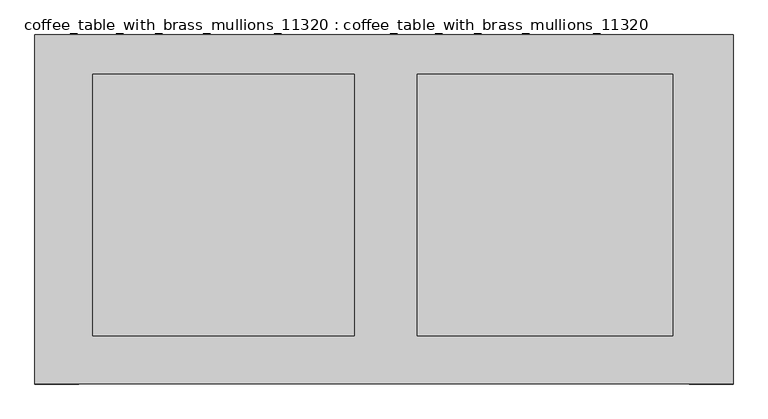
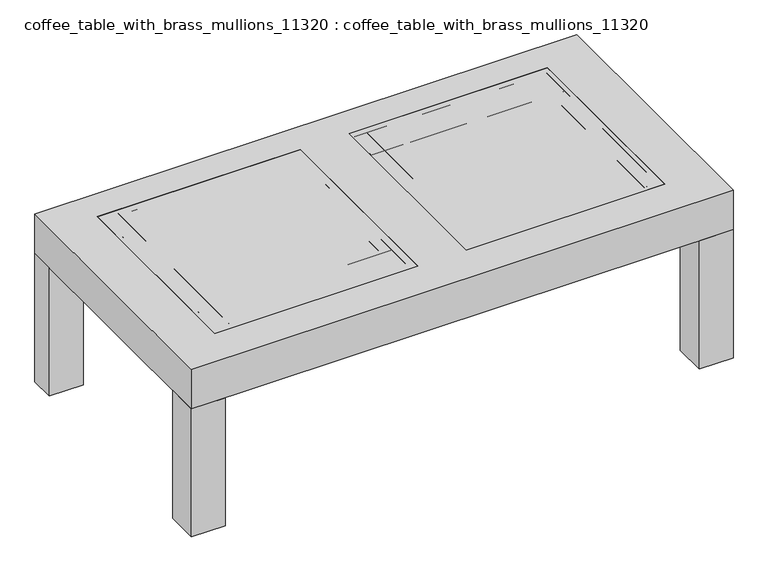
"""IFC4 building model written with IfcOpenShell, lengths in millimetres: proxy geometry, coffee_table_with_brass_mullions_11320 : coffee_table_with_brass_mullions_11320."""

from ifc_helpers import new_model, si_unit, frame, origin, place, context, project, spatial, polyline, outline, extrude, source, transform, mapped, element, save


def coffee_table_with_brass_mullions_11320_coffee_table_with_5962bef7(model_context):
    return source(origin(), model_context, "Body", "SweptSolid", [
        extrude(outline(polyline([(-1170.7012585, 125.388236), (-1246.9012585, 125.388236), (-1246.9012585, 198.4109722), (-1170.7012585, 198.4109722), (-1170.7012585, 125.388236)])), frame((0.0, 0.0, -180.3011333), z_axis=(0.0, 0.0, 1.0), x_axis=(1.0, 0.0, 0.0)), (0.0, 0.0, 1.0), 304.8),
        extrude(outline(polyline([(-27.7012585, 125.388236), (-103.9012585, 125.388236), (-103.9012585, 198.4109722), (-27.7012585, 198.4109722), (-27.7012585, 125.388236)])), frame((0.0, 0.0, -180.3011333), z_axis=(0.0, 0.0, 1.0), x_axis=(1.0, 0.0, 0.0)), (0.0, 0.0, 1.0), 304.8),
        extrude(outline(polyline([(-27.7012585, 678.8369834), (-103.9012585, 678.8369834), (-103.9012585, 734.988236), (-27.7012585, 734.988236), (-27.7012585, 678.8369834)])), frame((0.0, 0.0, -180.3011333), z_axis=(0.0, 0.0, 1.0), x_axis=(1.0, 0.0, 0.0)), (0.0, 0.0, 1.0), 304.8),
        extrude(outline(polyline([(-1170.7012585, 678.8369834), (-1246.9012585, 678.8369834), (-1246.9012585, 734.988236), (-1170.7012585, 734.988236), (-1170.7012585, 678.8369834)])), frame((0.0, 0.0, -180.3011333), z_axis=(0.0, 0.0, 1.0), x_axis=(1.0, 0.0, 0.0)), (0.0, 0.0, 1.0), 304.8),
        extrude(outline(polyline([(-27.7012585, 734.988236), (-27.7012585, 125.388236), (-1246.9012585, 125.388236), (-1246.9012585, 734.988236), (-27.7012585, 734.988236)]), holes=[polyline([(-689.0166493, 209.2726914), (-689.0166493, 666.4726914), (-1146.2166493, 666.4726914), (-1146.2166493, 209.2726914), (-689.0166493, 209.2726914)]), polyline([(-133.0123712, 209.2726914), (-133.0123712, 666.4726914), (-579.469964, 666.4726914), (-579.469964, 209.2726914), (-133.0123712, 209.2726914)])]), frame((0.0, 0.0, 124.4988667), z_axis=(0.0, 0.0, 1.0), x_axis=(1.0, 0.0, 0.0)), (0.0, 0.0, 1.0), 94.3180668),
        extrude(outline(polyline([(-689.0166493, 666.4726914), (-689.0166493, 209.2726914), (-1146.2166493, 209.2726914), (-1146.2166493, 666.4726914), (-689.0166493, 666.4726914)])), frame((0.0, 0.0, 197.8180045), z_axis=(0.0, 0.0, 1.0), x_axis=(1.0, 0.0, 0.0)), (0.0, 0.0, 1.0), 20.998929),
        extrude(outline(polyline([(-579.469964, 209.2726914), (-579.469964, 666.4726914), (-133.0123712, 666.4726914), (-133.0123712, 209.2726914), (-579.469964, 209.2726914)])), frame((0.0, 0.0, 197.8180045), z_axis=(0.0, 0.0, 1.0), x_axis=(1.0, 0.0, 0.0)), (0.0, 0.0, 1.0), 20.998929),
        extrude(outline(polyline([(-689.0166493, 209.2726914), (-1146.2166493, 209.2726914), (-1146.2166493, 666.4726914), (-689.0166493, 666.4726914), (-689.0166493, 209.2726914)]), holes=[polyline([(-706.0344683, 217.0199749), (-706.0344683, 648.8199749), (-1137.8344683, 648.8199749), (-1137.8344683, 217.0199749), (-706.0344683, 217.0199749)])]), frame((0.0, 0.0, 212.28904), z_axis=(0.0, 0.0, 1.0), x_axis=(1.0, 0.0, 0.0)), (0.0, 0.0, 1.0), 6.5278935),
        extrude(outline(polyline([(-723.165962, 215.6226914), (-729.515962, 215.6226914), (-729.515962, 672.8226914), (-723.165962, 672.8226914), (-723.165962, 215.6226914)])), frame((0.0, 0.0, 199.8285439), z_axis=(0.0, 0.0, 1.0), x_axis=(1.0, 0.0, 0.0)), (0.0, 0.0, 1.0), 18.9883896),
        extrude(outline(polyline([(-1099.4309107, 223.3699749), (-1105.7809107, 223.3699749), (-1105.7809107, 655.1699749), (-1099.4309107, 655.1699749), (-1099.4309107, 223.3699749)])), frame((0.0, 0.0, 199.8285439), z_axis=(0.0, 0.0, 1.0), x_axis=(1.0, 0.0, 0.0)), (0.0, 0.0, 1.0), 18.9883896),
        extrude(outline(polyline([(-706.0344683, 280.9206933), (-1137.8344683, 280.9206933), (-1137.8344683, 287.2706933), (-706.0344683, 287.2706933), (-706.0344683, 280.9206933)])), frame((0.0, 0.0, 212.28904), z_axis=(0.0, 0.0, 1.0), x_axis=(1.0, 0.0, 0.0)), (0.0, 0.0, 1.0), 6.5278935),
        extrude(outline(polyline([(-706.0344683, 580.4756876), (-1137.8344683, 580.4756876), (-1137.8344683, 586.8256876), (-706.0344683, 586.8256876), (-706.0344683, 580.4756876)])), frame((0.0, 0.0, 212.28904), z_axis=(0.0, 0.0, 1.0), x_axis=(1.0, 0.0, 0.0)), (0.0, 0.0, 1.0), 6.5278935),
        extrude(outline(polyline([(-133.0123712, 666.4726914), (-133.0123712, 209.2726914), (-579.469964, 209.2726914), (-579.469964, 666.4726914), (-133.0123712, 666.4726914)]), holes=[polyline([(-575.6343998, 219.3754253), (-143.8343998, 219.3754253), (-143.8343998, 651.1754253), (-575.6343998, 651.1754253), (-575.6343998, 219.3754253)])]), frame((0.0, 0.0, 197.8180045), z_axis=(0.0, 0.0, 1.0), x_axis=(1.0, 0.0, 0.0)), (0.0, 0.0, 1.0), 20.998929),
        extrude(outline(polyline([(-143.8343998, 586.8256876), (-143.8343998, 580.4756876), (-579.469964, 580.4756876), (-579.469964, 586.8256876), (-143.8343998, 586.8256876)])), frame((0.0, 0.0, 197.8180045), z_axis=(0.0, 0.0, 1.0), x_axis=(1.0, 0.0, 0.0)), (0.0, 0.0, 1.0), 20.998929),
        extrude(outline(polyline([(-143.8343998, 289.1161893), (-143.8343998, 282.7661893), (-575.6343998, 282.7661893), (-575.6343998, 289.1161893), (-143.8343998, 289.1161893)])), frame((0.0, 0.0, 197.8180045), z_axis=(0.0, 0.0, 1.0), x_axis=(1.0, 0.0, 0.0)), (0.0, 0.0, 1.0), 20.998929),
        extrude(outline(polyline([(-542.6218685, 651.1754253), (-542.6218685, 219.3754253), (-548.9718685, 219.3754253), (-548.9718685, 651.1754253), (-542.6218685, 651.1754253)])), frame((0.0, 0.0, 197.8180045), z_axis=(0.0, 0.0, 1.0), x_axis=(1.0, 0.0, 0.0)), (0.0, 0.0, 1.0), 20.998929),
        extrude(outline(polyline([(-167.3889038, 651.1754253), (-167.3889038, 219.3754253), (-173.7389038, 219.3754253), (-173.7389038, 651.1754253), (-167.3889038, 651.1754253)])), frame((0.0, 0.0, 197.8180045), z_axis=(0.0, 0.0, 1.0), x_axis=(1.0, 0.0, 0.0)), (0.0, 0.0, 1.0), 20.998929),
    ])


if __name__ == "__main__":
    model = new_model("IFC4")
    model_context = context("Model", 3, world=origin())
    ifc_project = project(units=[si_unit("LENGTHUNIT", "METRE", prefix="MILLI")], contexts=[model_context])
    site = spatial("IfcSite", under=ifc_project)
    building = spatial("IfcBuilding", under=site)
    placement = place(None, origin())
    coffee_table_with_brass_mullions_11320_coffee_table_with_shape = coffee_table_with_brass_mullions_11320_coffee_table_with_5962bef7(model_context)
    element("IfcBuildingElementProxy", 1, Name="coffee_table_with_brass_mullions_11320 : coffee_table_with_brass_mullions_11320", ObjectType="coffee_table_with_brass_mullions_11320 : coffee_table_with_brass_mullions_11320", at=placement, inside=building, context=model_context, shape_type="MappedRepresentation", body=[
        mapped(coffee_table_with_brass_mullions_11320_coffee_table_with_shape, transform((0.0, 0.0, 0.0), x_axis=(1.0, 0.0, 0.0), y_axis=(0.0, 1.0, 0.0), z_axis=(0.0, 0.0, 1.0))),
    ])
    save(model, "model.ifc")

# Revit data of these elements
# Type "coffee_table_with_brass_mullions_11320 : coffee_table_with_brass_mullions_11320"
#   Default Elevation = 0
# Element 1 (IfcBuildingElementProxy, "coffee_table_with_brass_mullions_11320 : coffee_table_with_brass_mullions_11320")
#   Materials on its faces: "Default Wall", "TABLE", "Glass", "Default"
# Materials
#   "Default Wall": colour RGB 128 128 128, transparency 0, Cost = 0
#   "TABLE": class "Generic", colour RGB 120 120 120, transparency 0, Cost = 0
#   "Glass": class "Glass", colour RGB 0 128 192, transparency 0.75, Description = "Soda Lime Glass", Cost = 0
#   "Default": colour RGB 127 127 127, transparency 0, Cost = 0
